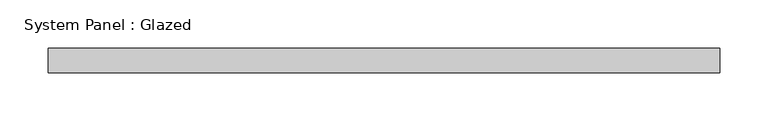
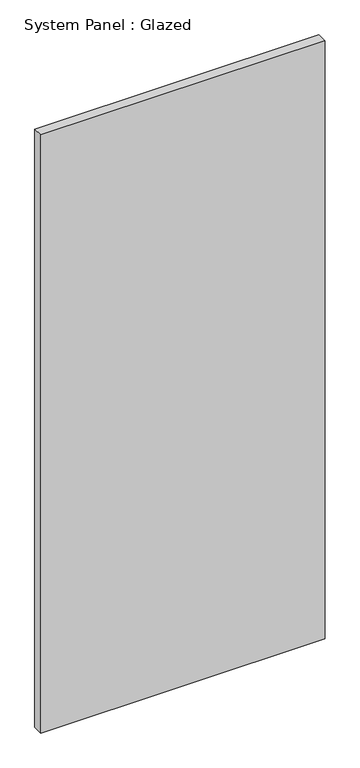
"""IFC4 building model written with IfcOpenShell, lengths in millimetres: plate geometry, System Panel : Glazed."""

from ifc_helpers import new_model, si_unit, origin, origin_with_axes, place, context, project, spatial, polyline, outline, extrude, source, transform, mapped, element, save


def system_panel_glazed_57682dc0(model_context):
    return source(origin(), model_context, "Body", "SweptSolid", [
        extrude(outline(polyline([(349.25, 19.05), (-349.25, 19.05), (-349.25, 44.45), (349.25, 44.45), (349.25, 19.05)])), origin_with_axes(), (0.0, 0.0, 1.0), 1553.4980219),
    ])


if __name__ == "__main__":
    model = new_model("IFC4")
    model_context = context("Model", 3, world=origin())
    ifc_project = project(units=[si_unit("LENGTHUNIT", "METRE", prefix="MILLI")], contexts=[model_context])
    site = spatial("IfcSite", under=ifc_project)
    building = spatial("IfcBuilding", under=site)
    placement = place(None, origin())
    system_panel_glazed_shape = system_panel_glazed_57682dc0(model_context)
    element("IfcPlate", 1, ObjectType="System Panel : Glazed", at=placement, inside=building, context=model_context, shape_type="MappedRepresentation", body=[
        mapped(system_panel_glazed_shape, transform((0.0, 0.0, 0.0), x_axis=(1.0, 0.0, 0.0), y_axis=(0.0, 1.0, 0.0), z_axis=(0.0, 0.0, 1.0))),
    ])
    save(model, "model.ifc")

# Revit data of these elements
# Type "System Panel : Glazed"
#   Construction Type Id = "GSP4R"
#   Analytic Construction = "1/8 in Pilkington single glazing"
#   Visual Light Transmittance = 0.9
#   Solar Heat Gain Coefficient = 0.86
#   Heat Transfer Coefficient (U) = 1.18115 BTU/(h·ft²·°F)
#   Define Thermal Properties by = 1
# Element 1 (IfcPlate, "System Panel : Glazed")
#   Materials on its faces: "Glass"
# Materials
#   "Glass": class "Glass", colour RGB 0 128 192, transparency 0.75, Description = "Soda Lime Glass", Cost = 0
